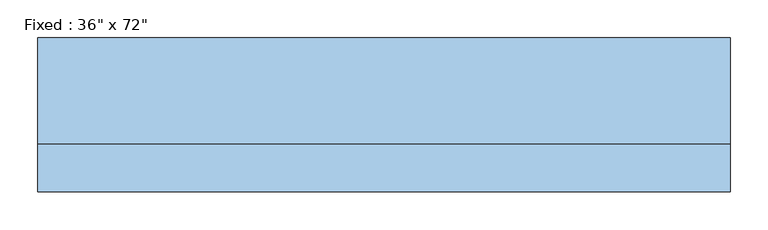
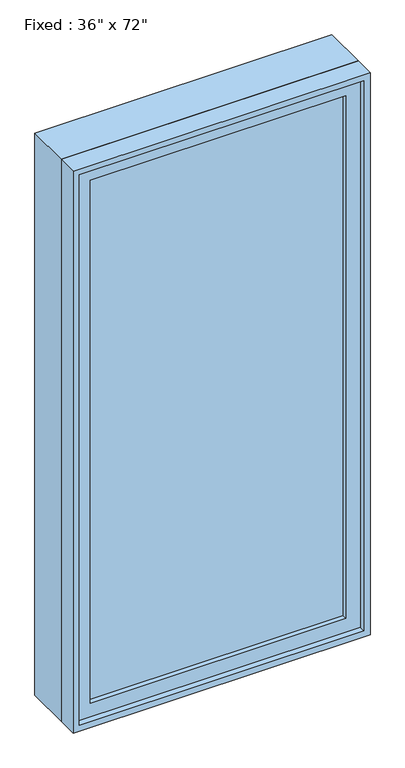
"""IFC4 building model written with IfcOpenShell, lengths in millimetres: window geometry."""

from ifc_helpers import new_model, si_unit, frame, origin, place, context, project, spatial, polyline, outline, extrude, source, transform, mapped, element, save


def window_750da936(model_context):
    return source(origin(), model_context, "Body", "SweptSolid", [
        extrude(outline(polyline([(355.6, -53.975), (355.6, -66.675), (-431.8, -66.675), (-431.8, -53.975), (355.6, -53.975)])), frame((0.0, 0.0, 368.3), z_axis=(0.0, 0.0, 1.0), x_axis=(1.0, 0.0, 0.0)), (0.0, 0.0, 1.0), 1701.8),
        extrude(outline(polyline([(2114.55, -476.25), (323.85, -476.25), (323.85, 400.05), (2114.55, 400.05), (2114.55, -476.25)]), holes=[polyline([(2070.1, -431.8), (2070.1, 355.6), (368.3, 355.6), (368.3, -431.8), (2070.1, -431.8)])]), frame((0.0, -82.55, 0.0), z_axis=(0.0, 1.0, 0.0), x_axis=(0.0, 0.0, 1.0)), (0.0, 0.0, 1.0), 44.45),
        extrude(outline(polyline([(2133.6, -495.3), (304.8, -495.3), (304.8, 419.1), (2133.6, 419.1), (2133.6, -495.3)]), holes=[polyline([(2101.85, -463.55), (2101.85, 387.35), (336.55, 387.35), (336.55, -463.55), (2101.85, -463.55)])]), frame((0.0, -38.1, 0.0), z_axis=(0.0, 1.0, 0.0), x_axis=(0.0, 0.0, 1.0)), (0.0, 0.0, 1.0), 139.7),
        extrude(outline(polyline([(2133.6, 419.1), (2133.6, -495.3), (304.8, -495.3), (304.8, 419.1), (2133.6, 419.1)]), holes=[polyline([(2114.55, 400.05), (323.85, 400.05), (323.85, -476.25), (2114.55, -476.25), (2114.55, 400.05)])]), frame((0.0, -101.6, 0.0), z_axis=(0.0, 1.0, 0.0), x_axis=(0.0, 0.0, 1.0)), (0.0, 0.0, 1.0), 63.5),
    ])


if __name__ == "__main__":
    model = new_model("IFC4")
    model_context = context("Model", 3, world=origin())
    ifc_project = project(units=[si_unit("LENGTHUNIT", "METRE", prefix="MILLI")], contexts=[model_context])
    site = spatial("IfcSite", under=ifc_project)
    building = spatial("IfcBuilding", under=site)
    placement = place(None, origin())
    window_shape = window_750da936(model_context)
    element("IfcWindow", 1, ObjectType="Fixed : 36\" x 72\"", at=placement, inside=building, context=model_context, shape_type="MappedRepresentation", body=[
        mapped(window_shape, transform((0.0, 0.0, 0.0), x_axis=(1.0, 0.0, 0.0), y_axis=(0.0, 1.0, 0.0), z_axis=(0.0, 0.0, 1.0))),
    ])
    save(model, "model.ifc")

# Revit data of these elements
# Type "Fixed : 36\" x 72\""
#   Type Mark = "9"
#   Construction Type Id = "GSP4R"
#   Assembly Code = "B2020100"
#   Analytic Construction = "1/8 in Pilkington single glazing"
#   Visual Light Transmittance = 0.9
#   Solar Heat Gain Coefficient = 0.78
#   Heat Transfer Coefficient (U) = 0.6496 BTU/(h·ft²·°F)
#   Height = 6' - 0"
#   Default Sill Height = 1' - 0"
#   Width = 3' - 0"
#   Window Inset = 0' - 0 3/4"
#   Define Thermal Properties by = 1
#   Glass Pane Material = Glass
#   Sash Material = Sash
#   Wall Closure = (empty or 0)
# Element 1 (IfcWindow, "Fixed : 36\" x 72\"")
#   Materials on its faces: "Sash", "Glass"
# Materials
#   "Glass": class "Glass", colour RGB 0 128 192, transparency 0.75, Description = "Soda Lime Glass", Cost = 0
#   "Sash": class "Wood", colour RGB 224 178 126, transparency 0
